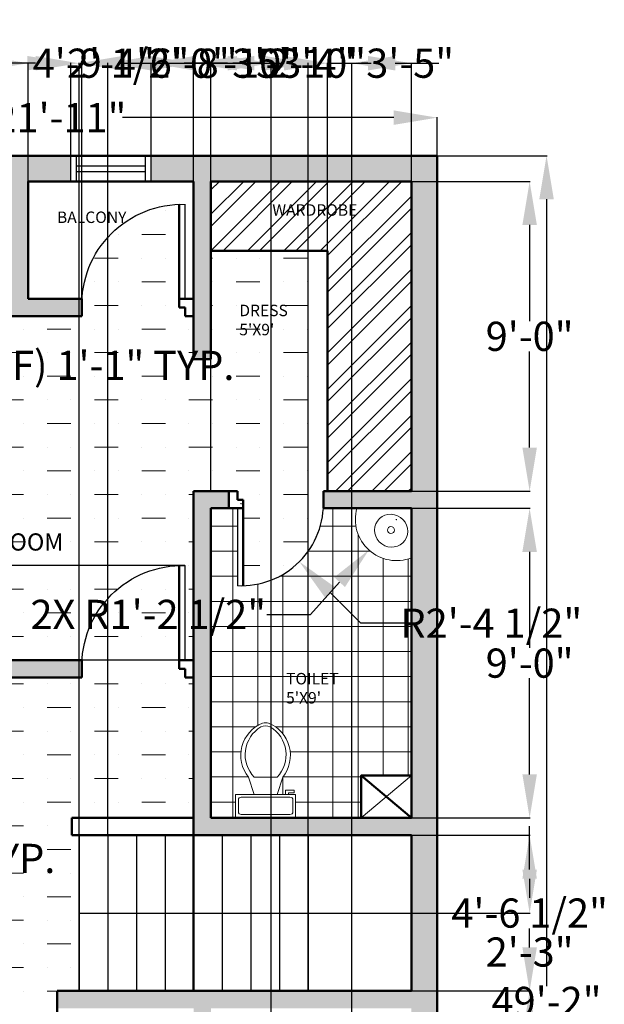
# Model space of a CAD drawing. Units: inches. Extents: x 26 to 14419, y 2 to 3479.
# Tile 9 of 9: x 14197 to 14401, y 3106 to 3449. Entities that reach past the tile are written whole.
import ezdxf

# ---------------------------------------------------------------- set-up
doc = ezdxf.new("R2010")
doc.units = ezdxf.units.IN
doc.header["$MEASUREMENT"] = 0
for name, color, linetype, lineweight in [('A-ANNO-DIMS', 2, 'Continuous', 18), ('A-AREA-IDEN', 7, 'Continuous', 18), ('A-DOOR', 4, 'Continuous', 25), ('A-FLOR-FIXT', 8, 'Continuous', 18), ('A-FLOR-PATT', 252, 'Continuous', 13), ('A-FLOR-STRS', 2, 'Continuous', 25), ('A-GLAZ', 3, 'Continuous', 25), ('A-WALL', 7, 'Continuous', 50)]:
    doc.layers.add(name, color=color, linetype=linetype, lineweight=lineweight)
doc.styles.get("Standard").update_dxf_attribs({"font": 'arial.ttf'})
doc.dimstyles.get("Standard").update_dxf_attribs({"dimtxt": 10.18, "dimasz": 15.18, "dimexe": 0.18, "dimexo": 0.0625, "dimgap": 0.09, "dimtad": 0, "dimtih": 1, "dimtoh": 1, "dimdec": 0, "dimzin": 0, "dimdsep": 46, "dimlunit": 3, "dimtxsty": 'Standard', "dimcen": 0.09, "dimadec": 0, "dimazin": 0, "dimtfac": 1, "dimtdec": 0, "dimtofl": 0, "dimtmove": 0, "dimatfit": 3, "dimfxl": 1, "dimtolj": 1, "dimtzin": 0, "dimarcsym": 0})

# ---------------------------------------------------------------- blocks, each defined once
blk = doc.blocks.new('*U2')
for p, q in [((9.5, -6), (9.5, -2)), ((-10, -8.5), (-8, -8.5)), ((-10, -9.5), (-10, -8.5)), ((-7, -9.5), (-10, -9.5)), ((-8, -8.5), (-8, -8)), ((-7, -8), (-7, -9.5)), ((-4, -8), (-6, -14)), ((4, -8), (6, -14)), ((4, -14), (-4, -14))]:
    blk.add_line(p, q)
blk.add_lwpolyline([(10.5, -8), (10.5, 0), (-10.5, 0), (-10.5, -8)], close=True)
for points in [[(-9.5, -2), (-9.5, -6)], [(8.5, -1), (-8.5, -1)], [(-8.5, -7), (8.5, -7)]]:
    blk.add_lwpolyline(points)
for centre, radius, start, end in [((-8.62, -1.88), 0.884, 81.8699, 188.1301), ((8.62, -1.88), 0.884, 351.8699, 98.1301), ((-8.62, -6.12), 0.884, 171.8699, 278.1301), ((8.62, -6.12), 0.884, 261.8699, 8.1301), ((3.52, -21.58), 12.17, 141.4691, 247.9714), ((4.2, -21.82), 11.33, 136.3677, 238.9468), ((-3.52, -21.58), 12.17, 292.0284, 38.5307), ((-4.2, -21.82), 11.33, 301.053, 43.6321), ((0, -27.88), 4, 245.7318, 294.2682), ((0, -29), 4, 254.8605, 285.1395)]:
    blk.add_arc(centre, radius, start, end)
blk = doc.blocks.new('*D8')
at = {"layer": 'A-ANNO-DIMS', "color": 0, "lineweight": -2, "transparency": 16777216}
for p, q in [((14079.64, 3401.78), (14079.64, 3415.17)), ((14094.82, 3414.99), (14189.53, 3414.99)), ((14327.46, 3414.99), (14232.76, 3414.99)), ((14342.64, 3401.78), (14342.64, 3415.17))]:
    blk.add_line(p, q, dxfattribs=at)
at = {"layer": 'A-ANNO-DIMS', "color": 0, "transparency": 16777216}
for points in [[(14094.82, 3417.52), (14094.82, 3412.46), (14079.64, 3414.99)], [(14327.46, 3417.52), (14327.46, 3412.46), (14342.64, 3414.99)]]:
    blk.add_solid(points, dxfattribs=at)
at = {"layer": 'Defpoints', "color": 0, "transparency": 16777216}
for p in [(14342.64, 3414.99), (14079.64, 3401.72), (14342.64, 3401.72)]:
    blk.add_point(p, dxfattribs=at)
at = {"layer": 'A-ANNO-DIMS', "color": 0, "transparency": 16777216, "insert": (14211.14, 3414.99), "char_height": 10.18, "attachment_point": 5}
blk.add_mtext('\\A1;21\'-11"', dxfattribs=at)
blk = doc.blocks.new('*D9')
at = {"layer": 'A-ANNO-DIMS', "color": 0, "lineweight": -2, "transparency": 16777216}
for p, q in [((14342.71, 3401.72), (14380.97, 3401.72)), ((14380.79, 3386.54), (14380.79, 3112.01)), ((14380.79, 2826.9), (14380.79, 3101.43)), ((14342.71, 2811.72), (14380.97, 2811.72))]:
    blk.add_line(p, q, dxfattribs=at)
at = {"layer": 'A-ANNO-DIMS', "color": 0, "transparency": 16777216}
for points in [[(14378.26, 3386.54), (14383.32, 3386.54), (14380.79, 3401.72)], [(14378.26, 2826.9), (14383.32, 2826.9), (14380.79, 2811.72)]]:
    blk.add_solid(points, dxfattribs=at)
at = {"layer": 'Defpoints', "color": 0, "transparency": 16777216}
for p in [(14342.64, 3401.72), (14342.64, 2811.72), (14380.79, 2811.72)]:
    blk.add_point(p, dxfattribs=at)
at = {"layer": 'A-ANNO-DIMS', "color": 0, "transparency": 16777216, "insert": (14380.79, 3106.72), "char_height": 10.18, "attachment_point": 5}
blk.add_mtext('\\A1;49\'-2"', dxfattribs=at)
blk = doc.blocks.new('DOOR-900')
blk.add_line((0, 3), (0, 36))
blk.add_arc((1, 1), 35.01, 358.3634, 91.6366)
blk = doc.blocks.new('*D33')
at = {"layer": 'A-ANNO-DIMS', "color": 0, "lineweight": -2, "transparency": 16777216}
for p, q in [((14111.8, 3187.7), (14121.24, 3187.7)), ((14121.06, 3172.52), (14121.06, 3163.38)), ((14121.06, 3140.7), (14121.06, 3149.84)), ((14111.8, 3125.52), (14121.24, 3125.52))]:
    blk.add_line(p, q, dxfattribs=at)
at = {"layer": 'A-ANNO-DIMS', "color": 0, "transparency": 16777216}
for points in [[(14118.53, 3172.52), (14123.59, 3172.52), (14121.06, 3187.7)], [(14118.53, 3140.7), (14123.59, 3140.7), (14121.06, 3125.52)]]:
    blk.add_solid(points, dxfattribs=at)
at = {"layer": 'Defpoints', "color": 0, "transparency": 16777216}
for p in [(14111.74, 3187.7), (14121.06, 3187.7), (14111.74, 3125.52)]:
    blk.add_point(p, dxfattribs=at)
at = {"layer": 'A-ANNO-DIMS', "color": 0, "transparency": 16777216, "insert": (14121.06, 3156.61), "char_height": 10.18, "attachment_point": 5}
blk.add_mtext('\\A1;3-SEAT SOFA (FF) 5\'-2" TYP.', dxfattribs=at)
blk = doc.blocks.new('*D37')
at = {"layer": 'A-ANNO-DIMS', "color": 0, "lineweight": -2, "transparency": 16777216}
for p, q in [((14081.32, 3328.58), (14066.14, 3328.58)), ((14096.5, 3330.45), (14096.5, 3328.4)), ((14109.33, 3330.45), (14109.33, 3328.4)), ((14124.51, 3328.58), (14139.69, 3328.58))]:
    blk.add_line(p, q, dxfattribs=at)
at = {"layer": 'A-ANNO-DIMS', "color": 0, "transparency": 16777216}
for points in [[(14081.32, 3331.11), (14081.32, 3326.05), (14096.5, 3328.58)], [(14124.51, 3331.11), (14124.51, 3326.05), (14109.33, 3328.58)]]:
    blk.add_solid(points, dxfattribs=at)
at = {"layer": 'Defpoints', "color": 0, "transparency": 16777216}
for p in [(14096.5, 3330.51), (14109.33, 3330.51), (14109.33, 3328.58)]:
    blk.add_point(p, dxfattribs=at)
at = {"layer": 'A-ANNO-DIMS', "color": 0, "transparency": 16777216, "insert": (14207.31, 3328.58), "char_height": 10.18, "attachment_point": 5}
blk.add_mtext('\\A1;LAMP (FF) 1\'-1" TYP.', dxfattribs=at)
blk = doc.blocks.new('*D103')
at = {"layer": 'A-ANNO-DIMS', "color": 0, "lineweight": -2, "transparency": 16777216}
for p, q in [((14333.71, 3164.72), (14375.07, 3164.72)), ((14374.89, 3149.54), (14374.89, 3142.9)), ((14374.89, 3125.55), (14374.89, 3132.19)), ((14333.71, 3110.37), (14375.07, 3110.37))]:
    blk.add_line(p, q, dxfattribs=at)
at = {"layer": 'A-ANNO-DIMS', "color": 0, "transparency": 16777216}
for points in [[(14372.36, 3149.54), (14377.42, 3149.54), (14374.89, 3164.72)], [(14372.36, 3125.55), (14377.42, 3125.55), (14374.89, 3110.37)]]:
    blk.add_solid(points, dxfattribs=at)
at = {"layer": 'Defpoints', "color": 0, "transparency": 16777216}
for p in [(14333.64, 3164.72), (14374.89, 3164.72), (14333.64, 3110.37)]:
    blk.add_point(p, dxfattribs=at)
at = {"layer": 'A-ANNO-DIMS', "color": 0, "transparency": 16777216, "insert": (14374.89, 3137.54), "char_height": 10.18, "attachment_point": 5}
blk.add_mtext('\\A1;4\'-6 1/2"', dxfattribs=at)
blk = doc.blocks.new('*D104')
at = {"layer": 'A-ANNO-DIMS', "color": 0, "lineweight": -2, "transparency": 16777216}
for p, q in [((14333.71, 3278.72), (14375.07, 3278.72)), ((14374.89, 3263.54), (14374.89, 3230.01)), ((14374.89, 3185.9), (14374.89, 3219.43)), ((14333.71, 3170.72), (14375.07, 3170.72))]:
    blk.add_line(p, q, dxfattribs=at)
at = {"layer": 'A-ANNO-DIMS', "color": 0, "transparency": 16777216}
for points in [[(14372.36, 3263.54), (14377.42, 3263.54), (14374.89, 3278.72)], [(14372.36, 3185.9), (14377.42, 3185.9), (14374.89, 3170.72)]]:
    blk.add_solid(points, dxfattribs=at)
at = {"layer": 'Defpoints', "color": 0, "transparency": 16777216}
for p in [(14333.64, 3278.72), (14374.89, 3278.72), (14333.64, 3170.72)]:
    blk.add_point(p, dxfattribs=at)
at = {"layer": 'A-ANNO-DIMS', "color": 0, "transparency": 16777216, "insert": (14374.89, 3224.72), "char_height": 10.18, "attachment_point": 5}
blk.add_mtext('\\A1;9\'-0"', dxfattribs=at)
blk = doc.blocks.new('*D105')
at = {"layer": 'A-ANNO-DIMS', "color": 0, "lineweight": -2, "transparency": 16777216}
for p, q in [((14333.71, 3392.72), (14375.07, 3392.72)), ((14374.89, 3377.54), (14374.89, 3344.01)), ((14374.89, 3299.9), (14374.89, 3333.43)), ((14333.71, 3284.72), (14375.07, 3284.72))]:
    blk.add_line(p, q, dxfattribs=at)
at = {"layer": 'A-ANNO-DIMS', "color": 0, "transparency": 16777216}
for points in [[(14372.36, 3377.54), (14377.42, 3377.54), (14374.89, 3392.72)], [(14372.36, 3299.9), (14377.42, 3299.9), (14374.89, 3284.72)]]:
    blk.add_solid(points, dxfattribs=at)
at = {"layer": 'Defpoints', "color": 0, "transparency": 16777216}
for p in [(14333.64, 3392.72), (14374.89, 3392.72), (14333.64, 3284.72)]:
    blk.add_point(p, dxfattribs=at)
at = {"layer": 'A-ANNO-DIMS', "color": 0, "transparency": 16777216, "insert": (14374.89, 3338.72), "char_height": 10.18, "attachment_point": 5}
blk.add_mtext('\\A1;9\'-0"', dxfattribs=at)
blk = doc.blocks.new('*D107')
at = {"layer": 'A-ANNO-DIMS', "color": 0, "lineweight": -2, "transparency": 16777216}
for p, q in [((14184.75, 3433.97), (14169.57, 3433.97)), ((14199.93, 3392.78), (14199.93, 3434.15)), ((14257.64, 3392.78), (14257.64, 3434.15)), ((14272.82, 3433.97), (14288, 3433.97))]:
    blk.add_line(p, q, dxfattribs=at)
at = {"layer": 'A-ANNO-DIMS', "color": 0, "transparency": 16777216}
for points in [[(14184.75, 3436.5), (14184.75, 3431.44), (14199.93, 3433.97)], [(14272.82, 3436.5), (14272.82, 3431.44), (14257.64, 3433.97)]]:
    blk.add_solid(points, dxfattribs=at)
at = {"layer": 'Defpoints', "color": 0, "transparency": 16777216}
for p in [(14257.64, 3433.97), (14199.93, 3392.72), (14257.64, 3392.72)]:
    blk.add_point(p, dxfattribs=at)
at = {"layer": 'A-ANNO-DIMS', "color": 0, "transparency": 16777216, "insert": (14228.78, 3433.97), "char_height": 10.18, "attachment_point": 5}
blk.add_mtext('\\A1;4\'-9 1/2"', dxfattribs=at)
blk = doc.blocks.new('*D108')
at = {"layer": 'A-ANNO-DIMS', "color": 0, "lineweight": -2, "transparency": 16777216}
for p, q in [((14263.64, 3392.78), (14263.64, 3434.15)), ((14278.82, 3433.97), (14281.07, 3433.97)), ((14318.46, 3433.97), (14316.22, 3433.97)), ((14333.64, 3392.78), (14333.64, 3434.15))]:
    blk.add_line(p, q, dxfattribs=at)
at = {"layer": 'A-ANNO-DIMS', "color": 0, "transparency": 16777216}
for points in [[(14278.82, 3436.5), (14278.82, 3431.44), (14263.64, 3433.97)], [(14318.46, 3436.5), (14318.46, 3431.44), (14333.64, 3433.97)]]:
    blk.add_solid(points, dxfattribs=at)
at = {"layer": 'Defpoints', "color": 0, "transparency": 16777216}
for p in [(14333.64, 3433.97), (14263.64, 3392.72), (14333.64, 3392.72)]:
    blk.add_point(p, dxfattribs=at)
at = {"layer": 'A-ANNO-DIMS', "color": 0, "transparency": 16777216, "insert": (14298.64, 3433.97), "char_height": 10.18, "attachment_point": 5}
blk.add_mtext('\\A1;5\'-10"', dxfattribs=at)
blk = doc.blocks.new('*D109')
at = {"layer": 'A-ANNO-DIMS', "color": 0, "lineweight": -2, "transparency": 16777216}
for p, q in [((14199.604862, 3433.969118), (14184.424862, 3433.969118)), ((14214.784862, 3401.781618), (14214.784862, 3434.149118)), ((14242.784862, 3401.781618), (14242.784862, 3434.149118)), ((14257.964862, 3433.969118), (14273.144862, 3433.969118))]:
    blk.add_line(p, q, dxfattribs=at)
at = {"layer": 'A-ANNO-DIMS', "color": 0, "transparency": 16777216}
for points in [[(14199.604862, 3436.499118), (14199.604862, 3431.439118), (14214.784862, 3433.969118)], [(14257.964862, 3436.499118), (14257.964862, 3431.439118), (14242.784862, 3433.969118)]]:
    blk.add_solid(points, dxfattribs=at)
at = {"layer": 'Defpoints', "color": 0, "transparency": 16777216}
for p in [(14242.784862, 3433.969118), (14214.784862, 3401.719118), (14242.784862, 3401.719118)]:
    blk.add_point(p, dxfattribs=at)
at = {"layer": 'A-ANNO-DIMS', "color": 0, "transparency": 16777216, "insert": (14228.784862, 3433.969118), "char_height": 10.18, "attachment_point": 5}
blk.add_mtext('\\A1;2\'-4"', dxfattribs=at)
blk = doc.blocks.new('*D112')
at = {"layer": 'A-ANNO-DIMS', "color": 0, "lineweight": -2, "transparency": 16777216}
for p, q in [((14269.46, 3433.97), (14254.28, 3433.97)), ((14284.64, 2882.78), (14284.64, 3434.15)), ((14312.82, 2882.82), (14312.82, 3434.15)), ((14328, 3433.97), (14343.18, 3433.97))]:
    blk.add_line(p, q, dxfattribs=at)
at = {"layer": 'A-ANNO-DIMS', "color": 0, "transparency": 16777216}
for points in [[(14269.46, 3436.5), (14269.46, 3431.44), (14284.64, 3433.97)], [(14328, 3436.5), (14328, 3431.44), (14312.82, 3433.97)]]:
    blk.add_solid(points, dxfattribs=at)
at = {"layer": 'Defpoints', "color": 0, "transparency": 16777216}
for p in [(14312.82, 3433.97), (14284.64, 2882.72), (14312.82, 2882.76)]:
    blk.add_point(p, dxfattribs=at)
at = {"layer": 'A-ANNO-DIMS', "color": 0, "transparency": 16777216, "insert": (14298.73, 3433.97), "char_height": 10.18, "attachment_point": 5}
blk.add_mtext('\\A1;2\'-4"', dxfattribs=at)
blk = doc.blocks.new('*D113')
at = {"layer": 'A-ANNO-DIMS', "color": 0, "lineweight": -2, "transparency": 16777216}
for p, q in [((14263.64, 3284.78), (14263.64, 3434.15)), ((14278.82, 3433.97), (14289.22, 3433.97)), ((14304.4, 3284.78), (14304.4, 3434.15)), ((14304.4, 3433.97), (14319.58, 3433.97))]:
    blk.add_line(p, q, dxfattribs=at)
at = {"layer": 'A-ANNO-DIMS', "color": 0, "transparency": 16777216}
for points in [[(14278.82, 3436.5), (14278.82, 3431.44), (14263.64, 3433.97)], [(14289.22, 3436.5), (14289.22, 3431.44), (14304.4, 3433.97)]]:
    blk.add_solid(points, dxfattribs=at)
at = {"layer": 'Defpoints', "color": 0, "transparency": 16777216}
for p in [(14304.4, 3433.97), (14263.64, 3284.72), (14304.4, 3284.72)]:
    blk.add_point(p, dxfattribs=at)
at = {"layer": 'A-ANNO-DIMS', "color": 0, "transparency": 16777216, "insert": (14333.19, 3433.97), "char_height": 10.18, "attachment_point": 5}
blk.add_mtext('\\A1;3\'-5"', dxfattribs=at)
blk = doc.blocks.new('*D114')
at = {"layer": 'A-ANNO-DIMS', "color": 0, "lineweight": -2, "transparency": 16777216}
for p, q in [((14218.64, 3345.81), (14218.64, 3434.15)), ((14233.82, 3433.97), (14242.46, 3433.97)), ((14257.64, 3345.81), (14257.64, 3434.15)), ((14257.64, 3433.97), (14272.82, 3433.97))]:
    blk.add_line(p, q, dxfattribs=at)
at = {"layer": 'A-ANNO-DIMS', "color": 0, "transparency": 16777216}
for points in [[(14233.82, 3436.5), (14233.82, 3431.44), (14218.64, 3433.97)], [(14242.46, 3436.5), (14242.46, 3431.44), (14257.64, 3433.97)]]:
    blk.add_solid(points, dxfattribs=at)
at = {"layer": 'Defpoints', "color": 0, "transparency": 16777216}
for p in [(14257.64, 3433.97), (14218.64, 3345.75), (14257.64, 3345.75)]:
    blk.add_point(p, dxfattribs=at)
at = {"layer": 'A-ANNO-DIMS', "color": 0, "transparency": 16777216, "insert": (14286.44, 3433.97), "char_height": 10.18, "attachment_point": 5}
blk.add_mtext('\\A1;3\'-3"', dxfattribs=at)
blk = doc.blocks.new('*D117')
at = {"layer": 'A-ANNO-DIMS', "color": 0, "lineweight": -2, "transparency": 16777216}
for p, q in [((14217.64, 3110.43), (14217.64, 3434.15)), ((14232.82, 3433.97), (14244, 3433.97)), ((14282.46, 3433.97), (14271.29, 3433.97)), ((14297.64, 3110.43), (14297.64, 3434.15))]:
    blk.add_line(p, q, dxfattribs=at)
at = {"layer": 'A-ANNO-DIMS', "color": 0, "transparency": 16777216}
for points in [[(14232.82, 3436.5), (14232.82, 3431.44), (14217.64, 3433.97)], [(14282.46, 3436.5), (14282.46, 3431.44), (14297.64, 3433.97)]]:
    blk.add_solid(points, dxfattribs=at)
at = {"layer": 'Defpoints', "color": 0, "transparency": 16777216}
for p in [(14297.64, 3433.97), (14217.64, 3110.37), (14297.64, 3110.37)]:
    blk.add_point(p, dxfattribs=at)
at = {"layer": 'A-ANNO-DIMS', "color": 0, "transparency": 16777216, "insert": (14257.64, 3433.97), "char_height": 10.18, "attachment_point": 5}
blk.add_mtext('\\A1;6\'-8"', dxfattribs=at)
blk = doc.blocks.new('*D118')
at = {"layer": 'A-ANNO-DIMS', "color": 0, "lineweight": -2, "transparency": 16777216}
for p, q in [((14202.46, 3433.97), (14187.28, 3433.97)), ((14217.64, 3164.78), (14217.64, 3434.15)), ((14227.64, 3164.78), (14227.64, 3434.15)), ((14242.82, 3433.97), (14258, 3433.97))]:
    blk.add_line(p, q, dxfattribs=at)
at = {"layer": 'A-ANNO-DIMS', "color": 0, "transparency": 16777216}
for points in [[(14202.46, 3436.5), (14202.46, 3431.44), (14217.64, 3433.97)], [(14242.82, 3436.5), (14242.82, 3431.44), (14227.64, 3433.97)]]:
    blk.add_solid(points, dxfattribs=at)
at = {"layer": 'Defpoints', "color": 0, "transparency": 16777216}
for p in [(14227.64, 3433.97), (14217.64, 3164.72), (14227.64, 3164.72)]:
    blk.add_point(p, dxfattribs=at)
at = {"layer": 'A-ANNO-DIMS', "color": 0, "transparency": 16777216, "insert": (14275.58, 3433.97), "char_height": 10.18, "attachment_point": 5}
blk.add_mtext('\\A1;0\'-10"', dxfattribs=at)
blk = doc.blocks.new('*D119')
at = {"layer": 'A-ANNO-DIMS', "color": 0, "lineweight": -2, "transparency": 16777216}
for p, q in [((14374.89, 3152.72), (14374.89, 3167.9)), ((14297.71, 3137.54), (14375.07, 3137.54)), ((14297.71, 3110.37), (14375.07, 3110.37)), ((14374.89, 3095.19), (14374.89, 3080.01))]:
    blk.add_line(p, q, dxfattribs=at)
at = {"layer": 'A-ANNO-DIMS', "color": 0, "transparency": 16777216}
for points in [[(14372.36, 3152.72), (14377.42, 3152.72), (14374.89, 3137.54)], [(14372.36, 3095.19), (14377.42, 3095.19), (14374.89, 3110.37)]]:
    blk.add_solid(points, dxfattribs=at)
at = {"layer": 'Defpoints', "color": 0, "transparency": 16777216}
for p in [(14297.64, 3137.54), (14374.89, 3137.54), (14297.64, 3110.37)]:
    blk.add_point(p, dxfattribs=at)
at = {"layer": 'A-ANNO-DIMS', "color": 0, "transparency": 16777216, "insert": (14374.89, 3123.96), "char_height": 10.18, "attachment_point": 5}
blk.add_mtext('\\A1;2\'-3"', dxfattribs=at)
blk = doc.blocks.new('*D120')
at = {"layer": 'A-ANNO-DIMS', "color": 0, "lineweight": -2, "transparency": 16777216}
for p, q in [((14047.39, 3258.75), (14047.39, 3273.93)), ((14047.39, 3273.93), (14062.57, 3273.93)), ((14254.58, 3258.75), (14047.21, 3258.75)), ((14047.39, 3240.93), (14047.39, 3243.57)), ((14257.58, 3225.75), (14047.21, 3225.75))]:
    blk.add_line(p, q, dxfattribs=at)
at = {"layer": 'A-ANNO-DIMS', "color": 0, "transparency": 16777216}
for points in [[(14044.86, 3243.57), (14049.92, 3243.57), (14047.39, 3258.75)], [(14044.86, 3240.93), (14049.92, 3240.93), (14047.39, 3225.75)]]:
    blk.add_solid(points, dxfattribs=at)
at = {"layer": 'Defpoints', "color": 0, "transparency": 16777216}
for p in [(14047.39, 3258.75), (14254.64, 3258.75), (14257.64, 3225.75)]:
    blk.add_point(p, dxfattribs=at)
at = {"layer": 'A-ANNO-DIMS', "color": 0, "transparency": 16777216, "insert": (14076.28, 3273.93), "char_height": 10.18, "attachment_point": 5}
blk.add_mtext('\\A1;2\'-9"', dxfattribs=at)
blk = doc.blocks.new('*D123')
at = {"layer": 'A-ANNO-DIMS', "color": 0, "lineweight": -2, "transparency": 16777216}
for p, q in [((14274.15, 3280.42), (14274.33, 3280.42)), ((14274.24, 3280.33), (14274.24, 3280.51)), ((14315.99, 3238.64), (14305.26, 3249.37)), ((14331.17, 3238.64), (14315.99, 3238.64))]:
    blk.add_line(p, q, dxfattribs=at)
at = {"layer": 'A-ANNO-DIMS', "color": 0, "transparency": 16777216}
blk.add_solid([(14307.05, 3251.16), (14303.47, 3247.59), (14294.53, 3260.11)], dxfattribs=at)
at = {"layer": 'Defpoints', "color": 0, "transparency": 16777216}
for p in [(14274.24, 3280.42), (14294.53, 3260.11)]:
    blk.add_point(p, dxfattribs=at)
at = {"layer": 'A-ANNO-DIMS', "color": 0, "transparency": 16777216, "insert": (14361.52, 3238.64), "char_height": 10.18, "attachment_point": 5}
blk.add_mtext('\\A1;R2\'-4 1/2"', dxfattribs=at)
blk = doc.blocks.new('*D124')
at = {"layer": 'A-ANNO-DIMS', "color": 0, "lineweight": -2, "transparency": 16777216}
for p, q in [((14328.38, 3274.85), (14328.56, 3274.85)), ((14328.47, 3274.76), (14328.47, 3274.94)), ((14298.37, 3241.72), (14308.58, 3252.96)), ((14283.19, 3241.72), (14298.37, 3241.72))]:
    blk.add_line(p, q, dxfattribs=at)
at = {"layer": 'A-ANNO-DIMS', "color": 0, "transparency": 16777216}
blk.add_solid([(14306.7, 3254.66), (14310.45, 3251.26), (14318.79, 3264.19)], dxfattribs=at)
at = {"layer": 'Defpoints', "color": 0, "transparency": 16777216}
for p in [(14328.47, 3274.85), (14318.79, 3264.19)]:
    blk.add_point(p, dxfattribs=at)
at = {"layer": 'A-ANNO-DIMS', "color": 0, "transparency": 16777216, "insert": (14241.81, 3241.72), "char_height": 10.18, "attachment_point": 5}
blk.add_mtext('\\A1;2X R1\'-2 1/2"', dxfattribs=at)

msp = doc.modelspace()

# ---------------------------------------------------------------- hatches: boundary and pattern name
at = {"layer": 'A-FLOR-PATT'}
h = msp.add_hatch(color=256, dxfattribs=at)
h.dxf.hatch_style = 1
h.paths.add_polyline_path([(13922.09, 3432), (13659.09, 3432), (13659.09, 2842), (13668.09, 2842), (13668.09, 2851), (13668.09, 2899), (13668.09, 2908), (13668.09, 3076), (13706.09, 3076), (13706.09, 3085), (13668.09, 3085), (13668.09, 3249), (13712.76, 3249), (13712.76, 3255), (13668.09, 3255), (13668.09, 3375), (13720.94, 3375), (13720.94, 3378, -0.017236), (13720.94, 3380), (13720.94, 3381), (13668.09, 3381), (13668.09, 3423), (13784.09, 3423), (13784.09, 3381), (13753.94, 3381), (13753.94, 3375), (13784.09, 3375), (13784.09, 3255), (13758.77, 3255), (13758.77, 3249), (13784.09, 3249), (13793.09, 3249), (13793.09, 3255), (13793.09, 3423), (13913.09, 3423), (13913.09, 3255), (13832.09, 3255), (13832.09, 3254, -0.014283), (13832.09, 3252), (13832.09, 3249), (13836.57, 3249), (13836.57, 3234), (13839.57, 3234, -0.017236), (13841.57, 3234), (13842.57, 3234), (13842.57, 3249), (13913.09, 3249), (13913.09, 3201), (13892.46, 3201), (13793.09, 3201), (13784.09, 3201), (13784.09, 3195), (13793.09, 3195), (13913.09, 3195), (13913.09, 3127), (13922.09, 3127)])
h.paths.add_polyline_path([(13922.09, 3013.5), (13913.09, 3013.5), (13913.09, 2908), (13892.09, 2908), (13892.09, 2899), (13913.09, 2899), (13913.09, 2851), (13793.09, 2851), (13784.09, 2851), (13784.09, 2842), (13922.09, 2842)], flags=17)
h.paths.add_polyline_path([(13793.09, 3085), (13784.09, 3085), (13784.09, 3076), (13784.09, 3071.08), (13784.09, 3066.17), (13784.09, 2908), (13784.09, 2899.07), (13793.09, 2899), (13802.09, 2899), (13814.09, 2899), (13814.09, 2908), (13793.09, 2908)], flags=17)
h.paths.add_polyline_path([(14342.64, 3401.72), (14242.78, 3401.72), (14242.78, 3392.72), (14257.64, 3392.72), (14257.64, 3351.75), (14257.64, 3345.75), (14257.64, 3330.73), (14263.64, 3330.73), (14263.64, 3392.72), (14333.64, 3392.72), (14333.64, 3284.72), (14302.92, 3284.72), (14302.92, 3281.72, -0.022645), (14302.92, 3279.12), (14302.92, 3278.72), (14333.64, 3278.72), (14333.64, 3170.72), (14316.1, 3170.72), (14263.64, 3170.72), (14263.64, 3278.72), (14269.92, 3278.72), (14269.92, 3284.72), (14263.64, 3284.72), (14257.64, 3284.72), (14257.64, 3225.75), (14257.64, 3219.75), (14257.64, 3164.72), (14333.64, 3164.72), (14333.64, 3110.37), (14210.01, 3110.37), (14210.01, 3104.37), (14257.64, 3104.37), (14257.64, 3024), (14263.64, 3024), (14263.64, 3039.72), (14263.64, 3104.37), (14333.64, 3104.37), (14333.64, 3045.72), (14333.64, 3039.72), (14333.64, 2967.72), (14296.64, 2967.72), (14296.64, 2964.72, -0.017236), (14296.64, 2962.72), (14296.64, 2961.72), (14333.64, 2961.72), (14333.64, 2882.72), (14312.64, 2882.72), (14312.64, 2873.72), (14333.64, 2873.72), (14333.64, 2820.72), (14333.64, 2811.72), (14342.64, 2811.72)])
h.paths.add_polyline_path([(14088.64, 3219.75), (14218.64, 3219.75), (14218.64, 3222.75, -0.014283), (14218.64, 3224.75), (14218.64, 3225.75), (14088.64, 3225.75), (14088.64, 3345.75), (14088.64, 3351.75), (14088.64, 3392.72), (14193.93, 3392.72), (14193.93, 3351.75), (14140.64, 3351.75), (14140.64, 3345.75), (14170.7, 3345.75), (14218.64, 3345.75), (14218.64, 3348.75, -0.014283), (14218.64, 3350.75), (14218.64, 3351.75), (14199.93, 3351.75), (14199.93, 3392.72), (14214.78, 3392.72), (14214.78, 3401.72), (14079.64, 3401.72), (14079.64, 2811.72), (14088.64, 2811.72), (14088.64, 2820.72), (14088.64, 2873.72), (14116.21, 2873.72), (14116.21, 2876.57), (14116.21, 2882.72), (14088.64, 2882.72), (14088.64, 3039.72), (14216.01, 3039.72), (14216.01, 3065.37), (14215.01, 3065.37, -0.014283), (14213.01, 3065.37), (14210.01, 3065.37), (14210.01, 3045.72), (14154.64, 3045.72), (14148.64, 3045.72), (14088.64, 3045.72)])
h.paths.add_polyline_path([(14284.64, 2882.72), (14263.64, 2882.72), (14263.64, 2961.72), (14263.64, 2967.72), (14257.64, 2967.72), (14257.64, 2956.69), (14257.64, 2916.18), (14257.64, 2882.72), (14249.61, 2882.72), (14249.61, 2873.72), (14284.64, 2873.72)], flags=17)
h.paths.add_polyline_path([(14202.78, 2882.72), (14189.55, 2882.72), (14189.55, 2879.95), (14189.55, 2873.72), (14202.78, 2873.72)], flags=17)
h = msp.add_hatch(dxfattribs=at)
h.set_pattern_fill('ANSI32', color=256, scale=24)
h.paths.add_polyline_path([(14333.64, 3392.72), (14263.64, 3392.72), (14263.64, 3368.55), (14304.4, 3368.55), (14304.4, 3284.72), (14333.64, 3284.72)])
h = msp.add_hatch(dxfattribs=at)
h.set_pattern_fill('MUDST', color=256, scale=33)
h.paths.add_polyline_path([(14304.4, 3368.55), (14263.64, 3368.55), (14263.64, 3330.73), (14257.64, 3330.73), (14257.64, 3345.75), (14254.64, 3345.75), (14254.64, 3348.75), (14252.64, 3348.75), (14252.64, 3384.75, 0.397579), (14218.64, 3350.75), (14218.64, 3345.75), (14170.7, 3345.75), (14170.7, 3274.26), (14114.64, 3274.26), (14114.64, 3345.75), (14088.64, 3345.75), (14088.64, 3225.75), (14114.67, 3225.75), (14114.67, 3239.54), (14174.56, 3239.54), (14174.56, 3225.75), (14218.69, 3225.75, -0.405865), (14254.64, 3258.75), (14254.64, 3225.75), (14257.64, 3225.75), (14257.64, 3284.72), (14263.64, 3284.72), (14272.92, 3284.72), (14272.92, 3281.72), (14274.92, 3281.72), (14274.92, 3251.72, 0.394163), (14302.92, 3279.12), (14302.92, 3284.72), (14304.4, 3284.72)])
h.paths.add_polyline_path([(14189.03, 3330.51), (14176.21, 3330.51), (14176.21, 3342.77), (14189.03, 3342.77)], flags=16)
h.paths.add_polyline_path([(14188.03, 3331.51), (14177.21, 3331.51), (14177.21, 3341.77), (14188.03, 3341.77)], flags=0)
h.paths.add_polyline_path([(14185.02, 3336.64, -1), (14180.21, 3336.64, -1)], flags=0)
h.paths.add_polyline_path([(14109.33, 3330.51), (14096.5, 3330.51), (14096.5, 3342.77), (14109.33, 3342.77)], flags=16)
h.paths.add_polyline_path([(14108.33, 3331.51), (14097.5, 3331.51), (14097.5, 3341.77), (14108.33, 3341.77)], flags=0)
h.paths.add_polyline_path([(14105.32, 3336.64, -1), (14100.51, 3336.64, -1)], flags=0)
h.paths.add_polyline_path([(14257.64, 3219.75), (14254.64, 3219.75), (14254.64, 3222.75), (14252.64, 3222.75), (14252.64, 3258.75, 0.397579), (14218.64, 3224.75), (14218.64, 3219.75), (14088.64, 3219.75), (14088.64, 3105.72), (14154.64, 3105.72), (14154.64, 3045.72), (14210.01, 3045.72), (14210.01, 3065.37), (14215.01, 3065.37, 0.397579), (14249.01, 3099.37), (14213.01, 3099.37), (14213.01, 3101.37), (14210.01, 3101.37), (14210.01, 3110.37), (14217.64, 3110.37), (14217.64, 3164.72), (14215.11, 3164.72), (14215.11, 3170.72), (14257.64, 3170.72)])
h.paths.add_polyline_path([(14174.2, 3192.28), (14172.21, 3192.28), (14172.21, 3190.47), (14113.94, 3190.47), (14113.94, 3192.28), (14112.02, 3192.28), (14112.02, 3207.65), (14113.94, 3207.65), (14174.2, 3207.65)], flags=16)
h.paths.add_polyline_path([(14132.26, 3203.31), (14132.26, 3205.54), (14153.01, 3205.54), (14153.01, 3203.31)], flags=0)
h.paths.add_polyline_path([(14139.45, 3178.77), (14139.45, 3144.03), (14124.04, 3144.03), (14124.04, 3178.77)], flags=16)
h.paths.add_polyline_path([(14138.45, 3177.77), (14138.45, 3145.03), (14125.04, 3145.03), (14125.04, 3177.77)], flags=0)
h.paths.add_polyline_path([(14127.62, 3154.26), (14127.69, 3154.32), (14127.65, 3154.8), (14127.17, 3154.71)], flags=0)
h.paths.add_polyline_path([(14137.62, 3155.43), (14138.07, 3155.38), (14137.86, 3155.74)], flags=0)
h.paths.add_polyline_path([(14134.11, 3152.76), (14134.62, 3152.52), (14134.75, 3152.98)], flags=0)
h.paths.add_polyline_path([(14134.97, 3149.61), (14135.06, 3149.3), (14135.3, 3149.21), (14134.97, 3149.61)], flags=0)
h.paths.add_polyline_path([(14129.06, 3148.22), (14128.85, 3148.19), (14128.88, 3147.91)], flags=0)
h.paths.add_polyline_path([(14129.76, 3149.73), (14129.77, 3149.7), (14129.81, 3149.73)], flags=0)
h.paths.add_polyline_path([(14129.81, 3152.94), (14129.51, 3152.8), (14129.91, 3152.74)], flags=0)
h.paths.add_polyline_path([(14129.97, 3154.13), (14131.4, 3152.09), (14132.47, 3152.75), (14132.58, 3152.96)], flags=0)
h.paths.add_polyline_path([(14131.76, 3158.63), (14131.62, 3158.74), (14131.67, 3158.49)], flags=0)
h.paths.add_polyline_path([(14133.11, 3151.99), (14133.11, 3152.01), (14133.11, 3151.99)], flags=0)
h.paths.add_polyline_path([(14135.18, 3148.48), (14135.04, 3148), (14135.53, 3147.73), (14135.69, 3148.25)], flags=0)
h.paths.add_polyline_path([(14111.74, 3127.44), (14109.92, 3127.44), (14109.92, 3125.52), (14094.56, 3125.52), (14094.56, 3127.44), (14094.56, 3187.7), (14109.92, 3187.7), (14109.92, 3185.71), (14111.74, 3185.71)], flags=16)
h.paths.add_polyline_path([(14098.89, 3166.51), (14098.89, 3145.76), (14096.67, 3145.76), (14096.67, 3166.51)], flags=0)
h.paths.add_polyline_path([(14107.98, 3191.64), (14092.66, 3191.64), (14092.66, 3205.45), (14107.98, 3205.45)], flags=16)
h.paths.add_polyline_path([(14102.61, 3192.64), (14102.72, 3192.57), (14102.74, 3192.64)], flags=0)
h.paths.add_polyline_path([(14101.15, 3198.79), (14101.66, 3198.55), (14101.79, 3199)], flags=0)
h.paths.add_polyline_path([(14105.37, 3201.99), (14105.29, 3202.26), (14105.04, 3201.95)], flags=0)
h.paths.add_polyline_path([(14102.01, 3195.63), (14102.11, 3195.33), (14102.34, 3195.23), (14102.02, 3195.64)], flags=0)
h.paths.add_polyline_path([(14102.22, 3194.5), (14102.08, 3194.03), (14102.57, 3193.75), (14102.73, 3194.27)], flags=0)
h.paths.add_polyline_path([(14096.1, 3194.24), (14095.89, 3194.22), (14095.92, 3193.93)], flags=0)
h.paths.add_polyline_path([(14096.81, 3195.75), (14096.81, 3195.72), (14096.85, 3195.75)], flags=0)
h.paths.add_polyline_path([(14094.74, 3200.21), (14094.69, 3200.82), (14094.21, 3200.74)], flags=0)
h.paths.add_polyline_path([(14096.86, 3198.97), (14096.55, 3198.82), (14096.95, 3198.77)], flags=0)
h.paths.add_polyline_path([(14097.01, 3200.16), (14098.44, 3198.11), (14099.51, 3198.78), (14099.62, 3198.98)], flags=0)
h.paths.add_polyline_path([(14098.8, 3204.66), (14098.66, 3204.77), (14098.71, 3204.51)], flags=0)
h.paths.add_polyline_path([(14100.15, 3198.02), (14100.15, 3198.03), (14100.15, 3198.02)], flags=0)
h.paths.add_polyline_path([(14257.64, 2967.72), (14263.64, 2967.72), (14266.64, 2967.72), (14296.64, 2967.72), (14304.52, 2967.72), (14304.52, 3072.04), (14263.64, 3072.04), (14263.64, 3039.72), (14263.64, 3024), (14257.64, 3024), (14257.64, 3104.37), (14216.01, 3104.37), (14216.01, 3101.37), (14249.01, 3101.37, -0.405865), (14216.01, 3065.41), (14216.01, 3039.72), (14088.64, 3039.72), (14088.64, 3034.24), (14107.2, 3034.24), (14107.2, 3010.33), (14088.64, 3010.33), (14088.64, 3001.38), (14176.64, 3001.38), (14176.64, 2931.05), (14088.64, 2931.05), (14088.64, 2926.95), (14107.2, 2926.95), (14107.2, 2903.04), (14088.64, 2903.04), (14088.64, 2882.72), (14116.21, 2882.72), (14116.21, 2876.57), (14151.84, 2876.57), (14151.84, 2882.72), (14189.55, 2882.72), (14257.64, 2882.72), (14257.64, 2916.18), (14244.9, 2916.18), (14244.9, 2956.69), (14257.64, 2956.69)])
h.paths.add_polyline_path([(14199.2, 2873.72), (14189.55, 2873.72), (14189.55, 2879.95), (14151.84, 2879.95), (14151.84, 2873.72), (14116.21, 2873.72), (14088.64, 2873.72), (14088.64, 2820.72), (14088.64, 2813.09), (14199.2, 2813.09)])
h.paths.add_polyline_path([(14272.13, 3336.81), (14293.39, 3336.81), (14293.39, 3351.73), (14272.13, 3351.73)], flags=24)
h.paths.add_polyline_path([(14208.53, 3375.98), (14237.24, 3375.98), (14237.24, 3384.22), (14208.53, 3384.22)], flags=25)
h.paths.add_polyline_path([(14136.68, 3250.57), (14220.54, 3250.57), (14220.54, 3272.96), (14136.68, 3272.96)], flags=24)
h.paths.add_polyline_path([(14121.4, 3116.81), (14182.4, 3116.81), (14182.4, 3131.73), (14121.4, 3131.73)], flags=24)
h.paths.add_polyline_path([(14268.29, 3033.43), (14289.54, 3033.43), (14289.54, 3048.36), (14268.29, 3048.36)], flags=24)
h.paths.add_polyline_path([(14151.68, 2960.42), (14207.58, 2960.42), (14207.58, 2975.35), (14151.68, 2975.35)], flags=25)
h.paths.add_polyline_path([(14128.74, 2839.15), (14157.44, 2839.15), (14157.44, 2847.39), (14128.74, 2847.39)], flags=24)
h = msp.add_hatch(dxfattribs=at)
h.set_pattern_fill('NET', color=256, scale=70)
h.paths.add_polyline_path([(14333.64, 3261.42, -0.616884), (14314.6, 3278.72), (14302.9, 3278.72, -0.410342), (14272.92, 3251.74), (14272.92, 3278.72), (14263.64, 3278.72), (14263.64, 3170.72), (14316.1, 3170.72), (14316.1, 3185.55), (14333.64, 3185.55)])
h.paths.add_polyline_path([(14288.74, 3184.95), (14286.74, 3178.95), (14289.74, 3178.95), (14289.74, 3180.45), (14292.74, 3180.45), (14292.74, 3179.45), (14290.74, 3179.45), (14290.74, 3178.95), (14293.24, 3178.95), (14293.24, 3170.95), (14272.24, 3170.95), (14272.24, 3178.95), (14278.74, 3178.95), (14276.74, 3184.95, -0.501323), (14281.7, 3203.81, -0.132891), (14283.79, 3203.81, -0.501317)], flags=16)
h.paths.add_polyline_path([(14286.74, 3184.95), (14278.74, 3184.95, -0.48008), (14281.1, 3202.48, -0.215004), (14284.38, 3202.48, -0.48008)], flags=0)
h.paths.add_polyline_path([(14292.24, 3176.95), (14292.24, 3172.95, -0.5), (14291.24, 3171.95), (14274.24, 3171.95, -0.5), (14273.24, 3172.95), (14273.24, 3176.95, -0.5), (14274.24, 3177.95), (14291.24, 3177.95, -0.5)], flags=0)

# ---------------------------------------------------------------- linework, layer by layer
at = {"layer": 'A-DOOR'}
msp.add_line((14272.92, 3278.72), (14272.92, 3251.72), dxfattribs=at)
msp.add_arc((14274.24, 3280.42), 28.71, 267.3628, 2.5945, dxfattribs=at)
at = {"layer": 'A-FLOR-FIXT'}
msp.add_line((14316.1, 3170.72), (14333.64, 3185.55), dxfattribs=at)
msp.add_circle((14326.5, 3271.13), 1.22, dxfattribs=at)
msp.add_arc((14328.47, 3274.85), 14.39, 164.4013, 291.0805, dxfattribs=at)
at = {"layer": 'A-FLOR-FIXT', "extrusion": (0, 0, -1)}
msp.add_ellipse((14326.56, 3270.9), major_axis=(-4.81, 3.38), ratio=0.960909, start_param=-6.283185, end_param=0, dxfattribs=at)
at = {"layer": 'A-FLOR-STRS'}
for p, q in [((14217.64, 3164.72), (14217.64, 3110.37)), ((14227.64, 3164.72), (14227.64, 3110.37)), ((14237.64, 3164.72), (14237.64, 3110.37)), ((14247.64, 3164.72), (14247.64, 3110.37)), ((14267.64, 3164.72), (14267.64, 3110.37)), ((14277.64, 3164.72), (14277.64, 3110.37)), ((14277.64, 3164.72), (14277.64, 3110.37)), ((14287.64, 3164.72), (14287.64, 3110.37)), ((14297.64, 3164.72), (14297.64, 3110.37)), ((14217.64, 3137.54), (14297.64, 3137.54))]:
    msp.add_line(p, q, dxfattribs=at)
at = {"layer": 'A-GLAZ'}
for p, q in [((14214.78, 3392.72), (14214.78, 3401.72)), ((14216.78, 3392.72), (14216.78, 3401.72)), ((14240.78, 3392.72), (14240.78, 3401.72)), ((14242.78, 3392.72), (14242.78, 3401.72)), ((14216.78, 3398.22), (14240.78, 3398.22)), ((14216.78, 3396.22), (14240.78, 3396.22))]:
    msp.add_line(p, q, dxfattribs=at)
at = {"layer": 'A-WALL'}
for p, q in [((14079.64, 3401.72), (14342.64, 3401.72)), ((14342.64, 3401.72), (14342.64, 2811.72)), ((14199.93, 3351.75), (14199.93, 3392.72)), ((14199.93, 3392.72), (14257.64, 3392.72)), ((14257.64, 3351.75), (14257.64, 3392.72)), ((14263.64, 3330.73), (14263.64, 3392.72)), ((14263.64, 3392.72), (14333.64, 3392.72)), ((14333.64, 3392.72), (14333.64, 3284.72)), ((14252.64, 3348.75), (14252.64, 3384.75)), ((14263.64, 3368.55), (14304.4, 3368.55)), ((14304.4, 3368.55), (14304.4, 3284.72)), ((14199.93, 3351.75), (14218.69, 3351.75)), ((14218.64, 3351.75), (14218.64, 3345.75)), ((14252.64, 3351.75), (14257.64, 3351.75)), ((14252.64, 3348.75), (14254.64, 3348.75)), ((14254.64, 3348.75), (14254.64, 3345.75)), ((14257.64, 3351.75), (14257.64, 3345.75)), ((14088.64, 3345.75), (14218.64, 3345.75)), ((14254.64, 3345.75), (14257.64, 3345.75)), ((14257.64, 3330.73), (14257.64, 3345.75)), ((14257.64, 3330.73), (14263.64, 3330.73)), ((14257.64, 3225.75), (14257.64, 3284.72)), ((14263.64, 3284.72), (14257.64, 3284.72)), ((14263.64, 3284.72), (14272.92, 3284.72)), ((14269.92, 3278.72), (14269.92, 3284.72)), ((14272.92, 3281.72), (14272.92, 3284.72)), ((14302.92, 3278.72), (14302.92, 3284.72)), ((14302.92, 3284.72), (14333.64, 3284.72)), ((14274.92, 3281.72), (14272.92, 3281.72)), ((14274.92, 3281.72), (14274.92, 3251.72)), ((14263.64, 3278.72), (14274.92, 3278.72)), ((14263.64, 3170.72), (14263.64, 3278.72)), ((14302.9, 3278.72), (14333.64, 3278.72)), ((14333.64, 3278.72), (14333.64, 3170.72)), ((14252.64, 3222.75), (14252.64, 3258.75)), ((14088.64, 3225.75), (14218.69, 3225.75)), ((14218.64, 3225.75), (14218.64, 3219.75)), ((14252.64, 3225.75), (14257.64, 3225.75)), ((14257.64, 3225.75), (14257.64, 3219.75)), ((14252.64, 3222.75), (14254.64, 3222.75)), ((14254.64, 3222.75), (14254.64, 3219.75)), ((14088.64, 3219.75), (14218.64, 3219.75)), ((14254.64, 3219.75), (14257.64, 3219.75)), ((14257.64, 3164.72), (14257.64, 3219.75)), ((14316.1, 3185.55), (14333.64, 3170.72)), ((14257.64, 3170.72), (14215.11, 3170.72)), ((14215.11, 3164.72), (14215.11, 3170.72)), ((14263.64, 3170.72), (14333.64, 3170.72)), ((14257.64, 3164.72), (14215.11, 3164.72)), ((14257.64, 3164.72), (14333.64, 3164.72)), ((14257.64, 3164.72), (14257.64, 3110.37)), ((14333.64, 3164.72), (14333.64, 3110.37)), ((14333.64, 3110.37), (14210.01, 3110.37)), ((14210.01, 3101.37), (14210.01, 3110.37))]:
    msp.add_line(p, q, dxfattribs=at)
msp.add_lwpolyline([(14333.64, 3170.72), (14316.1, 3170.72), (14316.1, 3185.55), (14333.64, 3185.55)], close=True, dxfattribs=at)

# ---------------------------------------------------------------- block references
at = {"layer": 'A-DOOR', "extrusion": (0, 0, -1), "zscale": -1}
for p in [(-14254.64, 3348.75), (-14254.64, 3222.75)]:
    msp.add_blockref('DOOR-900', p, dxfattribs=at)
at = {"layer": 'A-FLOR-FIXT', "rotation": 180}
msp.add_blockref('*U2', (14282.74, 3170.95), dxfattribs=at)

# ---------------------------------------------------------------- texts
at = {"layer": 'A-AREA-IDEN', "attachment_point": 1}
for s, width, insert, char_height in [('WARDROBE', 7.6086, (14285.1, 3384.77), 4), ('BALCONY', 7.6086, (14209.94, 3382.24), 4), ("DRESS\\P5'X9'", 7.6086, (14273.57, 3349.74), 4), ('MASTER BEDROOM\\P15\'1"X10\'', 89.8665, (14139.09, 3269.98), 6), ("TOILET\\P5'X9'", 7.6086, (14289.89, 3221.3), 4)]:
    msp.add_mtext_dynamic_manual_height_columns(s, width=width, gutter_width=1, heights=[0], dxfattribs=dict(at, insert=insert, char_height=char_height))

# ---------------------------------------------------------------- dimensions: what is measured, and where the dimension line sits
at = {"layer": 'A-ANNO-DIMS'}
for base, p1, p2, override, picture, middle in [((14257.64, 3433.97), (14199.93, 3392.72), (14257.64, 3392.72), {"dimdec": 1, "dimlfac": 1, "dimrnd": 0, "dimzin": 1, "dimdsep": 46, "dimlunit": 4, "dimfrac": 2}, '*D107', (14228.78, 3433.97)), ((14242.78, 3433.97), (14214.78, 3401.72), (14242.78, 3401.72), {"dimdec": 1, "dimlfac": 1, "dimrnd": 0, "dimzin": 1, "dimdsep": 46, "dimlunit": 4, "dimfrac": 2}, '*D109', (14228.78, 3433.97)), ((14227.64, 3433.97), (14217.64, 3164.72), (14227.64, 3164.72), {"dimdec": 1, "dimlfac": 1, "dimrnd": 0, "dimzin": 1, "dimdsep": 46, "dimlunit": 4, "dimfrac": 2}, '*D118', (14275.58, 3433.97)), ((14297.64, 3433.97), (14217.64, 3110.37), (14297.64, 3110.37), {"dimdec": 1, "dimlfac": 1, "dimrnd": 0, "dimzin": 1, "dimdsep": 46, "dimlunit": 4, "dimfrac": 2}, '*D117', (14257.64, 3433.97)), ((14257.64, 3433.97), (14218.64, 3345.75), (14257.64, 3345.75), {"dimdec": 1, "dimlfac": 1, "dimrnd": 0, "dimzin": 1, "dimdsep": 46, "dimlunit": 4, "dimfrac": 2}, '*D114', (14286.44, 3433.97)), ((14312.82, 3433.97), (14284.64, 2882.72), (14312.82, 2882.76), {"dimdec": 1, "dimlfac": 1, "dimrnd": 0, "dimzin": 1, "dimdsep": 46, "dimlunit": 4, "dimfrac": 2}, '*D112', (14298.73, 3433.97)), ((14333.64, 3433.97), (14263.64, 3392.72), (14333.64, 3392.72), {"dimdec": 1, "dimlfac": 1, "dimrnd": 0, "dimzin": 1, "dimdsep": 46, "dimlunit": 4, "dimfrac": 2}, '*D108', (14298.64, 3433.97)), ((14304.4, 3433.97), (14263.64, 3284.72), (14304.4, 3284.72), {"dimdec": 1, "dimlfac": 1, "dimrnd": 0, "dimzin": 1, "dimdsep": 46, "dimlunit": 4, "dimfrac": 2}, '*D113', (14333.19, 3433.97)), ((14342.64, 3414.99), (14079.64, 3401.72), (14342.64, 3401.72), {"dimclrd": 0, "dimclre": 0, "dimclrt": 0}, '*D8', (14211.14, 3414.99))]:
    dim = msp.add_linear_dim(base=base, p1=p1, p2=p2, dimstyle='Standard', override=override, dxfattribs=at)
    dim.commit()
    dim.dimension.update_dxf_attribs({"geometry": picture, "text_midpoint": middle})
for base, p1, p2, override, picture, middle in [((14380.79, 2811.72), (14342.64, 3401.72), (14342.64, 2811.72), {"dimclrd": 0, "dimclre": 0, "dimclrt": 0}, '*D9', (14380.79, 3106.72)), ((14374.89, 3392.72), (14333.64, 3284.72), (14333.64, 3392.72), {"dimdec": 1, "dimlfac": 1, "dimrnd": 0, "dimzin": 1, "dimdsep": 46, "dimlunit": 4, "dimfrac": 2}, '*D105', (14374.89, 3338.72)), ((14047.39, 3258.75), (14257.64, 3225.75), (14254.64, 3258.75), {"dimdec": 1, "dimlfac": 1, "dimrnd": 0, "dimzin": 1, "dimdsep": 46, "dimlunit": 4, "dimfrac": 2}, '*D120', (14076.28, 3273.93)), ((14374.89, 3278.72), (14333.64, 3170.72), (14333.64, 3278.72), {"dimdec": 1, "dimlfac": 1, "dimrnd": 0, "dimzin": 1, "dimdsep": 46, "dimlunit": 4, "dimfrac": 2}, '*D104', (14374.89, 3224.72)), ((14374.89, 3137.54), (14297.64, 3110.37), (14297.64, 3137.54), {"dimdec": 1, "dimlfac": 1, "dimrnd": 0, "dimzin": 1, "dimdsep": 46, "dimlunit": 4, "dimfrac": 2}, '*D119', (14374.89, 3123.96)), ((14374.8935, 3164.7191), (14333.6435, 3110.3671), (14333.6435, 3164.7191), {"dimdec": 1, "dimlfac": 1, "dimrnd": 0, "dimzin": 1, "dimdsep": 46, "dimlunit": 4, "dimfrac": 2}, '*D103', (14374.8935, 3137.5431))]:
    dim = msp.add_linear_dim(base=base, p1=p1, p2=p2, angle=90, dimstyle='Standard', override=override, dxfattribs=at)
    dim.commit()
    dim.dimension.update_dxf_attribs({"geometry": picture, "text_midpoint": middle})
dim = msp.add_linear_dim(base=(14109.33, 3328.58), p1=(14096.5, 3330.51), p2=(14109.33, 3330.51), text='LAMP (FF) <> TYP.', dimstyle='Standard', override={"dimdec": 1, "dimrnd": 0, "dimzin": 1, "dimlunit": 4, "dimfrac": 2}, dxfattribs=at)
dim.commit()
dim.dimension.update_dxf_attribs({"geometry": '*D37', "text_midpoint": (14207.31, 3328.58)})
dim = msp.add_radius_dim(center=(14274.24, 3280.42), mpoint=(14294.53, 3260.11), dimstyle='Standard', override={"dimdec": 1, "dimlfac": 1, "dimrnd": 0, "dimzin": 1, "dimdsep": 46, "dimlunit": 4, "dimfrac": 2}, dxfattribs=at)
dim.commit()
dim.dimension.update_dxf_attribs({"geometry": '*D123', "text_midpoint": (14361.52, 3238.64)})
dim = msp.add_radius_dim(center=(14328.47, 3274.85), mpoint=(14318.79, 3264.19), text='2X <>', dimstyle='Standard', override={"dimdec": 1, "dimlfac": 1, "dimrnd": 0, "dimzin": 1, "dimdsep": 46, "dimlunit": 4, "dimfrac": 2}, dxfattribs=at)
dim.commit()
dim.dimension.update_dxf_attribs({"geometry": '*D124', "text_midpoint": (14241.81, 3241.72)})
dim = msp.add_linear_dim(base=(14121.06, 3187.7), p1=(14111.74, 3125.52), p2=(14111.74, 3187.7), angle=90, text='3-SEAT SOFA (FF) <> TYP.', dimstyle='Standard', override={"dimdec": 1, "dimrnd": 0, "dimzin": 1, "dimlunit": 4, "dimfrac": 2}, dxfattribs=at)
dim.commit()
dim.dimension.update_dxf_attribs({"geometry": '*D33', "text_midpoint": (14121.06, 3156.61)})

doc.saveas('drawing.dxf')
